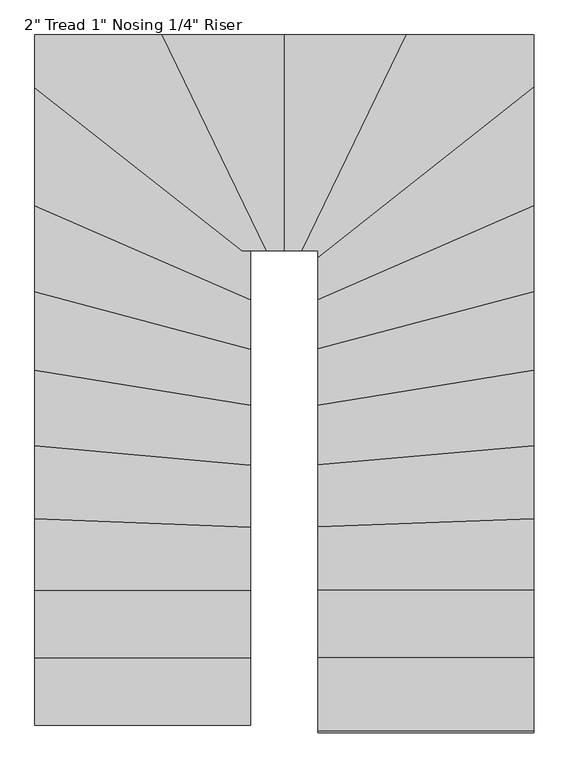
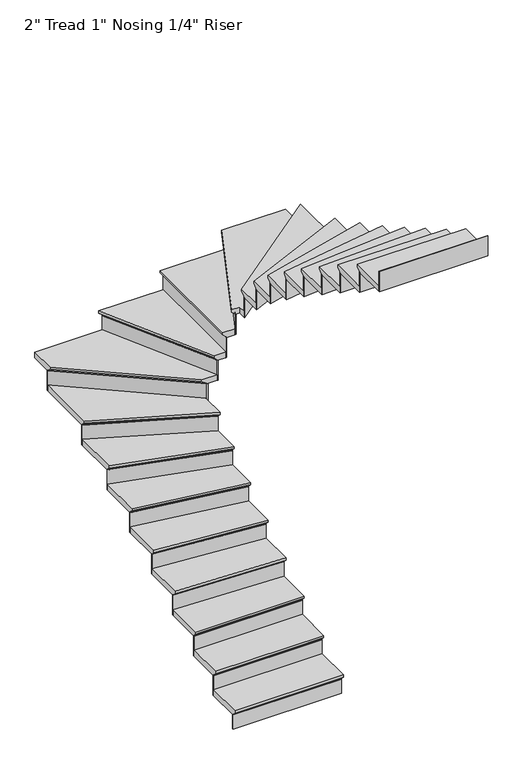
"""IFC4 building model written with IfcOpenShell, lengths in millimetres: stair flight geometry."""

from ifc_helpers import new_model, si_unit, origin, place, context, project, spatial, faceted_brep, source, transform, mapped, element, save


def stair_flight_77a7b7b7(model_context):
    return source(origin(), model_context, "Body", "Brep", [
        faceted_brep([(-5047.1987704, -4554.2130548, 25758.3214286), (-5047.1987704, -4554.2130548, 25777.3714286), (-5940.8822214, -4554.2130548, 25777.3714286), (-5940.8822214, -4554.2130548, 25758.3214286), (-5047.1987704, -4528.8130548, 25732.9214286), (-5940.8822214, -4528.8130548, 25732.9214286), (-5047.1987704, -4249.4130548, 25777.3714286), (-5940.8822214, -4249.4130548, 25777.3714286), (-5940.8822214, -4528.8130548, 25726.5714286), (-5940.8822214, -4249.4130548, 25726.5714286), (-5047.1987704, -4249.4130548, 25726.5714286), (-5047.1987704, -4528.8130548, 25726.5714286)], [[[0, 1, 2, 3]], [[4, 0, 3, 5]], [[2, 1, 6, 7]], [[8, 9, 10, 11]], [[2, 7, 9, 8, 5, 3]], [[8, 11, 4, 5]], [[6, 1, 0, 4, 11, 10]], [[7, 6, 10, 9]]]),
        faceted_brep([(-5047.1987704, -4528.8130548, 25726.5714286), (-5047.1987704, -4528.8130548, 25603.2), (-5047.1987704, -4522.4630548, 25603.2), (-5047.1987704, -4522.4630548, 25726.5714286), (-5940.8822214, -4528.8130548, 25726.5714286), (-5940.8822214, -4522.4630548, 25726.5714286), (-5940.8822214, -4522.4630548, 25603.2), (-5940.8822214, -4528.8130548, 25603.2)], [[[0, 1, 2, 3]], [[4, 5, 6, 7]], [[1, 0, 4, 7]], [[2, 1, 7, 6]], [[3, 2, 6, 5]], [[0, 3, 5, 4]]]),
        faceted_brep([(-5047.1987704, -4249.4130548, 25900.7428571), (-5047.1987704, -4249.4130548, 25726.5714286), (-5047.1987704, -4243.0630548, 25726.5714286), (-5047.1987704, -4243.0630548, 25900.7428571), (-5940.8822214, -4249.4130548, 25900.7428571), (-5940.8822214, -4243.0630548, 25900.7428571), (-5940.8822214, -4243.0630548, 25726.5714286), (-5940.8822214, -4249.4130548, 25726.5714286)], [[[0, 1, 2, 3]], [[4, 5, 6, 7]], [[1, 0, 4, 7]], [[2, 1, 7, 6]], [[3, 2, 6, 5]], [[0, 3, 5, 4]]]),
        faceted_brep([(-5940.8822214, -4274.8130548, 25951.5428571), (-5047.1987704, -4274.8130548, 25951.5428571), (-5047.1987704, -3970.0130548, 25951.5428571), (-5940.8822214, -3970.0130548, 25951.5428571), (-5940.8822214, -4249.4130548, 25900.7428571), (-5940.8822214, -3970.0130548, 25900.7428571), (-5047.1987704, -3970.0130548, 25900.7428571), (-5047.1987704, -4249.4130548, 25900.7428571), (-5940.8822214, -4249.4130548, 25907.0928571), (-5940.8822214, -4274.8130548, 25932.4928571), (-5047.1987704, -4249.4130548, 25907.0928571), (-5047.1987704, -4274.8130548, 25932.4928571)], [[[0, 1, 2, 3]], [[4, 5, 6, 7]], [[0, 3, 5, 4, 8, 9]], [[4, 7, 10, 8]], [[2, 1, 11, 10, 7, 6]], [[3, 2, 6, 5]], [[11, 1, 0, 9]], [[10, 11, 9, 8]]]),
        faceted_brep([(-5047.1987704, -3970.0130548, 26074.9142857), (-5047.1987704, -3970.0130548, 25900.7428571), (-5047.1987704, -3963.6630548, 25900.7428571), (-5047.1987704, -3963.6630548, 26074.9142857), (-5940.8822214, -3970.0130548, 26074.9142857), (-5940.8822214, -3963.6630548, 26074.9142857), (-5940.8822214, -3963.6630548, 25900.7428571), (-5940.8822214, -3970.0130548, 25900.7428571)], [[[0, 1, 2, 3]], [[4, 5, 6, 7]], [[1, 0, 4, 7]], [[2, 1, 7, 6]], [[3, 2, 6, 5]], [[0, 3, 5, 4]]]),
        faceted_brep([(-5940.8822214, -3995.4130548, 26125.7142857), (-5047.1987704, -3995.4130548, 26125.7142857), (-5047.1987704, -3707.9036879, 26125.7142857), (-5940.8822214, -3673.2843203, 26125.7142857), (-5940.8822214, -3970.0130548, 26074.9142857), (-5940.8822214, -3673.2843203, 26074.9142857), (-5047.1987704, -3707.9036879, 26074.9142857), (-5047.1987704, -3970.0130548, 26074.9142857), (-5940.8822214, -3970.0130548, 26081.2642857), (-5940.8822214, -3995.4130548, 26106.6642857), (-5047.1987704, -3970.0130548, 26081.2642857), (-5047.1987704, -3995.4130548, 26106.6642857)], [[[0, 1, 2, 3]], [[4, 5, 6, 7]], [[0, 3, 5, 4, 8, 9]], [[4, 7, 10, 8]], [[2, 1, 11, 10, 7, 6]], [[3, 2, 6, 5]], [[11, 1, 0, 9]], [[10, 11, 9, 8]]]),
        faceted_brep([(-5047.1987704, -3707.9036879, 26249.0857143), (-5047.1987704, -3707.9036879, 26074.9142857), (-5047.1987704, -3701.5489252, 26074.9142857), (-5047.1987704, -3701.5489252, 26249.0857143), (-5940.8822214, -3673.2843203, 26249.0857143), (-5940.8822214, -3666.9295576, 26249.0857143), (-5940.8822214, -3666.9295576, 26074.9142857), (-5940.8822214, -3673.2843203, 26074.9142857)], [[[0, 1, 2, 3]], [[4, 5, 6, 7]], [[1, 0, 4, 7]], [[2, 1, 7, 6]], [[3, 2, 6, 5]], [[0, 3, 5, 4]]]),
        faceted_brep([(-5940.8822214, -3698.703371, 26299.8857143), (-5047.1987704, -3733.3227386, 26299.8857143), (-5047.1987704, -3451.3234819, 26299.8857143), (-5940.8822214, -3370.89733, 26299.8857143), (-5940.8822214, -3673.2843203, 26249.0857143), (-5940.8822214, -3370.89733, 26249.0857143), (-5047.1987704, -3451.3234819, 26249.0857143), (-5047.1987704, -3707.9036879, 26249.0857143), (-5940.8822214, -3673.2843203, 26255.4357143), (-5940.8822214, -3698.703371, 26280.8357143), (-5047.1987704, -3707.9036879, 26255.4357143), (-5047.1987704, -3733.3227386, 26280.8357143)], [[[0, 1, 2, 3]], [[4, 5, 6, 7]], [[0, 3, 5, 4, 8, 9]], [[4, 7, 10, 8]], [[2, 1, 11, 10, 7, 6]], [[3, 2, 6, 5]], [[11, 1, 0, 9]], [[10, 11, 9, 8]]]),
        faceted_brep([(-5047.1987704, -3451.3234819, 26423.2571429), (-5047.1987704, -3451.3234819, 26249.0857143), (-5047.1987704, -3444.9478197, 26249.0857143), (-5047.1987704, -3444.9478197, 26423.2571429), (-5940.8822214, -3370.89733, 26423.2571429), (-5940.8822214, -3364.5216678, 26423.2571429), (-5940.8822214, -3364.5216678, 26249.0857143), (-5940.8822214, -3370.89733, 26249.0857143)], [[[0, 1, 2, 3]], [[4, 5, 6, 7]], [[1, 0, 4, 7]], [[2, 1, 7, 6]], [[3, 2, 6, 5]], [[0, 3, 5, 4]]]),
        faceted_brep([(-5940.8822214, -3396.3999789, 26474.0571429), (-5047.1987704, -3476.8261308, 26474.0571429), (-5047.1987704, -3203.4301079, 26474.0571429), (-5940.8822214, -3059.5417727, 26474.0571429), (-5940.8822214, -3370.89733, 26423.2571429), (-5940.8822214, -3059.5417727, 26423.2571429), (-5047.1987704, -3203.4301079, 26423.2571429), (-5047.1987704, -3451.3234819, 26423.2571429), (-5940.8822214, -3370.89733, 26429.6071429), (-5940.8822214, -3396.3999789, 26455.0071429), (-5047.1987704, -3451.3234819, 26429.6071429), (-5047.1987704, -3476.8261308, 26455.0071429)], [[[0, 1, 2, 3]], [[4, 5, 6, 7]], [[0, 3, 5, 4, 8, 9]], [[4, 7, 10, 8]], [[2, 1, 11, 10, 7, 6]], [[3, 2, 6, 5]], [[11, 1, 0, 9]], [[10, 11, 9, 8]]]),
        faceted_brep([(-5047.1987704, -3203.4301079, 26597.4285714), (-5047.1987704, -3203.4301079, 26423.2571429), (-5047.1987704, -3196.9983292, 26423.2571429), (-5047.1987704, -3196.9983292, 26597.4285714), (-5940.8822214, -3059.5417727, 26597.4285714), (-5940.8822214, -3053.109994, 26597.4285714), (-5940.8822214, -3053.109994, 26423.2571429), (-5940.8822214, -3059.5417727, 26423.2571429)], [[[0, 1, 2, 3]], [[4, 5, 6, 7]], [[1, 0, 4, 7]], [[2, 1, 7, 6]], [[3, 2, 6, 5]], [[0, 3, 5, 4]]]),
        faceted_brep([(-5940.8822214, -3085.2688872, 26648.2285714), (-5047.1987704, -3229.1572224, 26648.2285714), (-5047.1987704, -2970.3553609, 26648.2285714), (-5940.8822214, -2732.7052783, 26648.2285714), (-5940.8822214, -3059.5417727, 26597.4285714), (-5940.8822214, -2732.7052783, 26597.4285714), (-5047.1987704, -2970.3553609, 26597.4285714), (-5047.1987704, -3203.4301079, 26597.4285714), (-5940.8822214, -3059.5417727, 26603.7785714), (-5940.8822214, -3085.2688872, 26629.1785714), (-5047.1987704, -3203.4301079, 26603.7785714), (-5047.1987704, -3229.1572224, 26629.1785714)], [[[0, 1, 2, 3]], [[4, 5, 6, 7]], [[0, 3, 5, 4, 8, 9]], [[4, 7, 10, 8]], [[2, 1, 11, 10, 7, 6]], [[3, 2, 6, 5]], [[11, 1, 0, 9]], [[10, 11, 9, 8]]]),
        faceted_brep([(-5047.1987704, -2970.3553609, 26771.6), (-5047.1987704, -2970.3553609, 26597.4285714), (-5047.1987704, -2963.7846771, 26597.4285714), (-5047.1987704, -2963.7846771, 26771.6), (-5940.8822214, -2732.7052783, 26771.6), (-5940.8822214, -2726.1345945, 26771.6), (-5940.8822214, -2726.1345945, 26597.4285714), (-5940.8822214, -2732.7052783, 26597.4285714)], [[[0, 1, 2, 3]], [[4, 5, 6, 7]], [[1, 0, 4, 7]], [[2, 1, 7, 6]], [[3, 2, 6, 5]], [[0, 3, 5, 4]]]),
        faceted_brep([(-5940.8822214, -2758.9880136, 26822.4), (-5047.1987704, -2996.6380961, 26822.4), (-5047.1987704, -2765.8050203, 26822.4), (-5940.8822214, -2375.5896532, 26822.4), (-5940.8822214, -2732.7052783, 26771.6), (-5940.8822214, -2375.5896532, 26771.6), (-5047.1987704, -2765.8050203, 26771.6), (-5047.1987704, -2970.3553609, 26771.6), (-5940.8822214, -2732.7052783, 26777.95), (-5940.8822214, -2758.9880136, 26803.35), (-5047.1987704, -2970.3553609, 26777.95), (-5047.1987704, -2996.6380961, 26803.35)], [[[0, 1, 2, 3]], [[4, 5, 6, 7]], [[0, 3, 5, 4, 8, 9]], [[4, 7, 10, 8]], [[2, 1, 11, 10, 7, 6]], [[3, 2, 6, 5]], [[11, 1, 0, 9]], [[10, 11, 9, 8]]]),
        faceted_brep([(-5047.1987704, -2765.8050203, 26945.7714286), (-5047.1987704, -2765.8050203, 26771.6), (-5047.1987704, -2758.8760908, 26771.6), (-5047.1987704, -2758.8760908, 26945.7714286), (-5940.8822214, -2375.5896532, 26945.7714286), (-5940.8822214, -2368.6607237, 26945.7714286), (-5940.8822214, -2368.6607237, 26771.6), (-5940.8822214, -2375.5896532, 26771.6)], [[[0, 1, 2, 3]], [[4, 5, 6, 7]], [[1, 0, 4, 7]], [[2, 1, 7, 6]], [[3, 2, 6, 5]], [[0, 3, 5, 4]]]),
        faceted_brep([(-5940.8822214, -2403.3053713, 26996.5714286), (-5047.1987704, -2793.5207384, 26996.5714286), (-5047.1987704, -2590.8424524, 26996.5714286), (-5040.8038639, -2590.8424524, 26996.5714286), (-5940.8822214, -1882.1944717, 26996.5714286), (-5940.8822214, -2375.5896532, 26945.7714286), (-5940.8822214, -1882.1944717, 26945.7714286), (-5040.8038639, -2590.8424524, 26945.7714286), (-5047.1987704, -2590.8424524, 26945.7714286), (-5047.1987704, -2765.8050203, 26945.7714286), (-5940.8822214, -2375.5896532, 26952.1214286), (-5940.8822214, -2403.3053713, 26977.5214286), (-5047.1987704, -2765.8050203, 26952.1214286), (-5047.1987704, -2793.5207384, 26977.5214286)], [[[0, 1, 2, 3, 4]], [[5, 6, 7, 8, 9]], [[0, 4, 6, 5, 10, 11]], [[5, 9, 12, 10]], [[2, 1, 13, 12, 9, 8]], [[4, 3, 7, 6]], [[13, 1, 0, 11]], [[12, 13, 11, 10]], [[3, 2, 8, 7]]]),
        faceted_brep([(-5040.8038639, -2590.8424524, 27119.9428571), (-5040.8038639, -2590.8424524, 26945.7714286), (-5030.5387554, -2590.8424524, 26945.7714286), (-5030.5387554, -2590.8424524, 27119.9428571), (-5940.8822214, -1882.1944717, 27119.9428571), (-5940.8822214, -1874.1125661, 27119.9428571), (-5940.8822214, -1874.1125661, 26945.7714286), (-5940.8822214, -1882.1944717, 26945.7714286)], [[[0, 1, 2, 3]], [[4, 5, 6, 7]], [[1, 0, 4, 7]], [[2, 1, 7, 6]], [[3, 2, 6, 5]], [[0, 3, 5, 4]]]),
        faceted_brep([(-5384.6489457, -1697.1590014, 27170.7428571), (-5940.8822214, -1697.1590014, 27170.7428571), (-5940.8822214, -1914.5220945, 27170.7428571), (-5081.8642978, -2590.8424524, 27170.7428571), (-4952.3566185, -2590.8424524, 27170.7428571), (-5940.8822214, -1697.1590014, 27119.9428571), (-5384.6489457, -1697.1590014, 27119.9428571), (-4952.3566185, -2590.8424524, 27119.9428571), (-5040.8038639, -2590.8424524, 27119.9428571), (-5940.8822214, -1882.1944717, 27119.9428571), (-5940.8822214, -1882.1944717, 27126.2928571), (-5940.8822214, -1914.5220945, 27151.6928571), (-5040.8038639, -2590.8424524, 27126.2928571), (-5081.8642978, -2590.8424524, 27151.6928571)], [[[0, 1, 2, 3, 4]], [[5, 6, 7, 8, 9]], [[1, 0, 6, 5]], [[2, 1, 5, 9, 10, 11]], [[9, 8, 12, 10]], [[4, 3, 13, 12, 8, 7]], [[0, 4, 7, 6]], [[13, 3, 2, 11]], [[12, 13, 11, 10]]]),
        faceted_brep([(-4952.3566185, -2590.8424524, 27294.1142857), (-4952.3566185, -2590.8424524, 27119.9428571), (-4945.3027294, -2590.8424524, 27119.9428571), (-4945.3027294, -2590.8424524, 27294.1142857), (-5384.6489457, -1697.1590014, 27294.1142857), (-5377.5950566, -1697.1590014, 27294.1142857), (-5377.5950566, -1697.1590014, 27119.9428571), (-5384.6489457, -1697.1590014, 27119.9428571)], [[[0, 1, 2, 3]], [[4, 5, 6, 7]], [[1, 0, 4, 7]], [[2, 1, 7, 6]], [[3, 2, 6, 5]], [[0, 3, 5, 4]]]),
        faceted_brep([(-5412.8645022, -1697.1590014, 27344.9142857), (-4980.5721749, -2590.8424524, 27344.9142857), (-4882.0987704, -2590.8424524, 27344.9142857), (-4882.0987706, -1697.1590014, 27344.9142857), (-5384.6489457, -1697.1590014, 27294.1142857), (-4882.0987706, -1697.1590014, 27294.1142857), (-4882.0987704, -2590.8424524, 27294.1142857), (-4952.3566185, -2590.8424524, 27294.1142857), (-5384.6489457, -1697.1590014, 27300.4642857), (-5412.8645022, -1697.1590014, 27325.8642857), (-4952.3566185, -2590.8424524, 27300.4642857), (-4980.5721749, -2590.8424524, 27325.8642857)], [[[0, 1, 2, 3]], [[4, 5, 6, 7]], [[0, 3, 5, 4, 8, 9]], [[4, 7, 10, 8]], [[3, 2, 6, 5]], [[11, 1, 0, 9]], [[10, 11, 9, 8]], [[2, 1, 11, 10, 7, 6]]]),
        faceted_brep([(-4882.0987704, -2590.8424524, 27468.2857143), (-4882.0987704, -2590.8424524, 27294.1142857), (-4875.7487704, -2590.8424524, 27294.1142857), (-4875.7487704, -2590.8424524, 27468.2857143), (-4882.0987706, -1697.1590014, 27468.2857143), (-4875.7487706, -1697.1590014, 27468.2857143), (-4875.7487706, -1697.1590014, 27294.1142857), (-4882.0987706, -1697.1590014, 27294.1142857)], [[[0, 1, 2, 3]], [[4, 5, 6, 7]], [[1, 0, 4, 7]], [[2, 1, 7, 6]], [[3, 2, 6, 5]], [[0, 3, 5, 4]]]),
        faceted_brep([(-4907.4987706, -1697.1590014, 27519.0857143), (-4907.4987704, -2590.8424524, 27519.0857143), (-4806.2098095, -2590.8424524, 27519.0857143), (-4373.9174828, -1697.1590014, 27519.0857143), (-4882.0987706, -1697.1590014, 27468.2857143), (-4373.9174828, -1697.1590014, 27468.2857143), (-4806.2098095, -2590.8424524, 27468.2857143), (-4882.0987704, -2590.8424524, 27468.2857143), (-4882.0987706, -1697.1590014, 27474.6357143), (-4907.4987706, -1697.1590014, 27500.0357143), (-4882.0987704, -2590.8424524, 27474.6357143), (-4907.4987704, -2590.8424524, 27500.0357143)], [[[0, 1, 2, 3]], [[4, 5, 6, 7]], [[0, 3, 5, 4, 8, 9]], [[4, 7, 10, 8]], [[2, 1, 11, 10, 7, 6]], [[3, 2, 6, 5]], [[11, 1, 0, 9]], [[10, 11, 9, 8]]]),
        faceted_brep([(-4806.2098095, -2590.8424524, 27642.4571429), (-4806.2098095, -2590.8424524, 27468.2857143), (-4799.1559204, -2590.8424524, 27468.2857143), (-4799.1559204, -2590.8424524, 27642.4571429), (-4373.9174828, -1697.1590014, 27642.4571429), (-4366.8635937, -1697.1590014, 27642.4571429), (-4366.8635937, -1697.1590014, 27468.2857143), (-4373.9174828, -1697.1590014, 27468.2857143)], [[[0, 1, 2, 3]], [[4, 5, 6, 7]], [[1, 0, 4, 7]], [[2, 1, 7, 6]], [[3, 2, 6, 5]], [[0, 3, 5, 4]]]),
        faceted_brep([(-3874.1153195, -1946.8497166, 27693.2571429), (-3874.1153195, -1697.1590014, 27693.2571429), (-4402.1330392, -1697.1590014, 27693.2571429), (-4834.4253659, -2590.8424524, 27693.2571429), (-4767.7987704, -2590.8424524, 27693.2571429), (-4767.7987704, -2650.4628721, 27693.2571429), (-3874.1153195, -1697.1590014, 27642.4571429), (-3874.1153195, -1946.8497166, 27642.4571429), (-4767.7987704, -2650.4628721, 27642.4571429), (-4767.7987704, -2590.8424524, 27642.4571429), (-4806.2098095, -2590.8424524, 27642.4571429), (-4373.9174828, -1697.1590014, 27642.4571429), (-4806.2098095, -2590.8424524, 27648.8071429), (-4373.9174828, -1697.1590014, 27648.8071429), (-4834.4253659, -2590.8424524, 27674.2071429), (-4402.1330392, -1697.1590014, 27674.2071429)], [[[0, 1, 2, 3, 4, 5]], [[6, 7, 8, 9, 10, 11]], [[1, 0, 7, 6]], [[11, 10, 12, 13]], [[4, 3, 14, 12, 10, 9]], [[5, 4, 9, 8]], [[0, 5, 8, 7]], [[14, 3, 2, 15]], [[12, 14, 15, 13]], [[2, 1, 6, 11, 13, 15]]]),
        faceted_brep([(-4767.7987704, -2650.4628721, 27816.6285714), (-4767.7987704, -2650.4628721, 27642.4571429), (-4767.7987704, -2658.5447778, 27642.4571429), (-4767.7987704, -2658.5447778, 27816.6285714), (-3874.1153195, -1946.8497166, 27816.6285714), (-3874.1153195, -1954.9316222, 27816.6285714), (-3874.1153195, -1954.9316222, 27642.4571429), (-3874.1153195, -1946.8497166, 27642.4571429)], [[[0, 1, 2, 3]], [[4, 5, 6, 7]], [[1, 0, 4, 7]], [[2, 1, 7, 6]], [[3, 2, 6, 5]], [[0, 3, 5, 4]]]),
        faceted_brep([(-3874.1153195, -1914.5220938, 27867.4285714), (-4767.7987704, -2618.1352494, 27867.4285714), (-4767.7987704, -2821.2364563, 27867.4285714), (-3874.1153195, -2431.0210889, 27867.4285714), (-3874.1153195, -1946.8497166, 27816.6285714), (-3874.1153195, -2431.0210889, 27816.6285714), (-4767.7987704, -2821.2364563, 27816.6285714), (-4767.7987704, -2650.4628721, 27816.6285714), (-3874.1153195, -1946.8497166, 27822.9785714), (-3874.1153195, -1914.5220938, 27848.3785714), (-4767.7987704, -2650.4628721, 27822.9785714), (-4767.7987704, -2618.1352494, 27848.3785714)], [[[0, 1, 2, 3]], [[4, 5, 6, 7]], [[0, 3, 5, 4, 8, 9]], [[4, 7, 10, 8]], [[2, 1, 11, 10, 7, 6]], [[3, 2, 6, 5]], [[11, 1, 0, 9]], [[10, 11, 9, 8]]]),
        faceted_brep([(-4767.7987704, -2821.2364563, 27990.8), (-4767.7987704, -2821.2364563, 27816.6285714), (-4767.7987704, -2828.1653858, 27816.6285714), (-4767.7987704, -2828.1653858, 27990.8), (-3874.1153195, -2431.0210889, 27990.8), (-3874.1153195, -2437.9500185, 27990.8), (-3874.1153195, -2437.9500185, 27816.6285714), (-3874.1153195, -2431.0210889, 27816.6285714)], [[[0, 1, 2, 3]], [[4, 5, 6, 7]], [[1, 0, 4, 7]], [[2, 1, 7, 6]], [[3, 2, 6, 5]], [[0, 3, 5, 4]]]),
        faceted_brep([(-3874.1153195, -2403.3053709, 28041.6), (-4767.7987704, -2793.5207382, 28041.6), (-4767.7987704, -3022.9208311, 28041.6), (-3874.1153195, -2785.2707484, 28041.6), (-3874.1153195, -2431.0210889, 27990.8), (-3874.1153195, -2785.2707484, 27990.8), (-4767.7987704, -3022.9208311, 27990.8), (-4767.7987704, -2821.2364563, 27990.8), (-3874.1153195, -2431.0210889, 27997.15), (-3874.1153195, -2403.3053709, 28022.55), (-4767.7987704, -2821.2364563, 27997.15), (-4767.7987704, -2793.5207382, 28022.55)], [[[0, 1, 2, 3]], [[4, 5, 6, 7]], [[0, 3, 5, 4, 8, 9]], [[4, 7, 10, 8]], [[2, 1, 11, 10, 7, 6]], [[3, 2, 6, 5]], [[11, 1, 0, 9]], [[10, 11, 9, 8]]]),
        faceted_brep([(-4767.7987704, -3022.9208311, 28164.9714286), (-4767.7987704, -3022.9208311, 27990.8), (-4767.7987704, -3029.4915149, 27990.8), (-4767.7987704, -3029.4915149, 28164.9714286), (-3874.1153195, -2785.2707484, 28164.9714286), (-3874.1153195, -2791.8414322, 28164.9714286), (-3874.1153195, -2791.8414322, 27990.8), (-3874.1153195, -2785.2707484, 27990.8)], [[[0, 1, 2, 3]], [[4, 5, 6, 7]], [[1, 0, 4, 7]], [[2, 1, 7, 6]], [[3, 2, 6, 5]], [[0, 3, 5, 4]]]),
        faceted_brep([(-3874.1153195, -2758.9880132, 28215.7714286), (-4767.7987704, -2996.6380959, 28215.7714286), (-4767.7987704, -3254.8843368, 28215.7714286), (-3874.1153195, -3110.9960015, 28215.7714286), (-3874.1153195, -2785.2707484, 28164.9714286), (-3874.1153195, -3110.9960015, 28164.9714286), (-4767.7987704, -3254.8843368, 28164.9714286), (-4767.7987704, -3022.9208311, 28164.9714286), (-3874.1153195, -2785.2707484, 28171.3214286), (-3874.1153195, -2758.9880132, 28196.7214286), (-4767.7987704, -3022.9208311, 28171.3214286), (-4767.7987704, -2996.6380959, 28196.7214286)], [[[0, 1, 2, 3]], [[4, 5, 6, 7]], [[0, 3, 5, 4, 8, 9]], [[4, 7, 10, 8]], [[2, 1, 11, 10, 7, 6]], [[3, 2, 6, 5]], [[11, 1, 0, 9]], [[10, 11, 9, 8]]]),
        faceted_brep([(-4767.7987704, -3254.8843368, 28339.1428571), (-4767.7987704, -3254.8843368, 28164.9714286), (-4767.7987704, -3261.3161154, 28164.9714286), (-4767.7987704, -3261.3161154, 28339.1428571), (-3874.1153195, -3110.9960015, 28339.1428571), (-3874.1153195, -3117.4277801, 28339.1428571), (-3874.1153195, -3117.4277801, 28164.9714286), (-3874.1153195, -3110.9960015, 28164.9714286)], [[[0, 1, 2, 3]], [[4, 5, 6, 7]], [[1, 0, 4, 7]], [[2, 1, 7, 6]], [[3, 2, 6, 5]], [[0, 3, 5, 4]]]),
        faceted_brep([(-3874.1153195, -3085.2688869, 28389.9428571), (-4767.7987704, -3229.1572222, 28389.9428571), (-4767.7987704, -3502.3287795, 28389.9428571), (-3874.1153195, -3421.9026274, 28389.9428571), (-3874.1153195, -3110.9960015, 28339.1428571), (-3874.1153195, -3421.9026274, 28339.1428571), (-4767.7987704, -3502.3287795, 28339.1428571), (-4767.7987704, -3254.8843368, 28339.1428571), (-3874.1153195, -3110.9960015, 28345.4928571), (-3874.1153195, -3085.2688869, 28370.8928571), (-4767.7987704, -3254.8843368, 28345.4928571), (-4767.7987704, -3229.1572222, 28370.8928571)], [[[0, 1, 2, 3]], [[4, 5, 6, 7]], [[0, 3, 5, 4, 8, 9]], [[4, 7, 10, 8]], [[2, 1, 11, 10, 7, 6]], [[3, 2, 6, 5]], [[11, 1, 0, 9]], [[10, 11, 9, 8]]]),
        faceted_brep([(-4767.7987704, -3502.3287795, 28513.3142857), (-4767.7987704, -3502.3287795, 28339.1428571), (-4767.7987704, -3508.7044417, 28339.1428571), (-4767.7987704, -3508.7044417, 28513.3142857), (-3874.1153195, -3421.9026274, 28513.3142857), (-3874.1153195, -3428.2782897, 28513.3142857), (-3874.1153195, -3428.2782897, 28339.1428571), (-3874.1153195, -3421.9026274, 28339.1428571)], [[[0, 1, 2, 3]], [[4, 5, 6, 7]], [[1, 0, 4, 7]], [[2, 1, 7, 6]], [[3, 2, 6, 5]], [[0, 3, 5, 4]]]),
        faceted_brep([(-3874.1153195, -3396.3999786, 28564.1142857), (-4767.7987704, -3476.8261306, 28564.1142857), (-4767.7987704, -3758.7417891, 28564.1142857), (-3874.1153195, -3724.1224215, 28564.1142857), (-3874.1153195, -3421.9026274, 28513.3142857), (-3874.1153195, -3724.1224215, 28513.3142857), (-4767.7987704, -3758.7417891, 28513.3142857), (-4767.7987704, -3502.3287795, 28513.3142857), (-3874.1153195, -3421.9026274, 28519.6642857), (-3874.1153195, -3396.3999786, 28545.0642857), (-4767.7987704, -3502.3287795, 28519.6642857), (-4767.7987704, -3476.8261306, 28545.0642857)], [[[0, 1, 2, 3]], [[4, 5, 6, 7]], [[0, 3, 5, 4, 8, 9]], [[4, 7, 10, 8]], [[2, 1, 11, 10, 7, 6]], [[3, 2, 6, 5]], [[11, 1, 0, 9]], [[10, 11, 9, 8]]]),
        faceted_brep([(-4767.7987704, -3758.7417891, 28687.4857143), (-4767.7987704, -3758.7417891, 28513.3142857), (-4767.7987704, -3765.0965518, 28513.3142857), (-4767.7987704, -3765.0965518, 28687.4857143), (-3874.1153195, -3724.1224215, 28687.4857143), (-3874.1153195, -3730.4771842, 28687.4857143), (-3874.1153195, -3730.4771842, 28513.3142857), (-3874.1153195, -3724.1224215, 28513.3142857)], [[[0, 1, 2, 3]], [[4, 5, 6, 7]], [[1, 0, 4, 7]], [[2, 1, 7, 6]], [[3, 2, 6, 5]], [[0, 3, 5, 4]]]),
        faceted_brep([(-3874.1153195, -3698.7033708, 28738.2857143), (-4767.7987704, -3733.3227384, 28738.2857143), (-4767.7987704, -4020.8130546, 28738.2857143), (-3874.1153195, -4020.8130546, 28738.2857143), (-3874.1153195, -3724.1224215, 28687.4857143), (-3874.1153195, -4020.8130546, 28687.4857143), (-4767.7987704, -4020.8130546, 28687.4857143), (-4767.7987704, -3758.7417891, 28687.4857143), (-3874.1153195, -3724.1224215, 28693.8357143), (-3874.1153195, -3698.7033708, 28719.2357143), (-4767.7987704, -3758.7417891, 28693.8357143), (-4767.7987704, -3733.3227384, 28719.2357143)], [[[0, 1, 2, 3]], [[4, 5, 6, 7]], [[0, 3, 5, 4, 8, 9]], [[4, 7, 10, 8]], [[2, 1, 11, 10, 7, 6]], [[3, 2, 6, 5]], [[11, 1, 0, 9]], [[10, 11, 9, 8]]]),
        faceted_brep([(-4767.7987704, -4020.8130546, 28861.6571429), (-4767.7987704, -4020.8130546, 28687.4857143), (-4767.7987704, -4027.1630546, 28687.4857143), (-4767.7987704, -4027.1630546, 28861.6571429), (-3874.1153195, -4020.8130546, 28861.6571429), (-3874.1153195, -4027.1630546, 28861.6571429), (-3874.1153195, -4027.1630546, 28687.4857143), (-3874.1153195, -4020.8130546, 28687.4857143)], [[[0, 1, 2, 3]], [[4, 5, 6, 7]], [[1, 0, 4, 7]], [[2, 1, 7, 6]], [[3, 2, 6, 5]], [[0, 3, 5, 4]]]),
        faceted_brep([(-3874.1153195, -3995.4130546, 28912.4571429), (-4767.7987704, -3995.4130546, 28912.4571429), (-4767.7987704, -4300.2130546, 28912.4571429), (-3874.1153195, -4300.2130546, 28912.4571429), (-3874.1153195, -4020.8130546, 28861.6571429), (-3874.1153195, -4300.2130546, 28861.6571429), (-4767.7987704, -4300.2130546, 28861.6571429), (-4767.7987704, -4020.8130546, 28861.6571429), (-3874.1153195, -4020.8130546, 28868.0071429), (-3874.1153195, -3995.4130546, 28893.4071429), (-4767.7987704, -4020.8130546, 28868.0071429), (-4767.7987704, -3995.4130546, 28893.4071429)], [[[0, 1, 2, 3]], [[4, 5, 6, 7]], [[0, 3, 5, 4, 8, 9]], [[4, 7, 10, 8]], [[2, 1, 11, 10, 7, 6]], [[3, 2, 6, 5]], [[11, 1, 0, 9]], [[10, 11, 9, 8]]]),
        faceted_brep([(-4767.7987704, -4300.2130546, 29035.8285714), (-4767.7987704, -4300.2130546, 28861.6571429), (-4767.7987704, -4306.5630546, 28861.6571429), (-4767.7987704, -4306.5630546, 29035.8285714), (-3874.1153195, -4300.2130546, 29035.8285714), (-3874.1153195, -4306.5630546, 29035.8285714), (-3874.1153195, -4306.5630546, 28861.6571429), (-3874.1153195, -4300.2130546, 28861.6571429)], [[[0, 1, 2, 3]], [[4, 5, 6, 7]], [[1, 0, 4, 7]], [[2, 1, 7, 6]], [[3, 2, 6, 5]], [[0, 3, 5, 4]]]),
        faceted_brep([(-4767.7987704, -4579.6130546, 29210.0), (-4767.7987704, -4579.6130546, 29035.8285714), (-4767.7987704, -4585.9630546, 29035.8285714), (-4767.7987704, -4585.9630546, 29210.0), (-3874.1153195, -4579.6130546, 29210.0), (-3874.1153195, -4585.9630546, 29210.0), (-3874.1153195, -4585.9630546, 29035.8285714), (-3874.1153195, -4579.6130546, 29035.8285714)], [[[0, 1, 2, 3]], [[4, 5, 6, 7]], [[1, 0, 4, 7]], [[2, 1, 7, 6]], [[3, 2, 6, 5]], [[0, 3, 5, 4]]]),
        faceted_brep([(-3874.1153195, -4274.8130546, 29086.6285714), (-4767.7987704, -4274.8130546, 29086.6285714), (-4767.7987704, -4579.6130546, 29086.6285714), (-3874.1153195, -4579.6130546, 29086.6285714), (-3874.1153195, -4300.2130546, 29035.8285714), (-3874.1153195, -4579.6130546, 29035.8285714), (-4767.7987704, -4579.6130546, 29035.8285714), (-4767.7987704, -4300.2130546, 29035.8285714), (-3874.1153195, -4300.2130546, 29042.1785714), (-3874.1153195, -4274.8130546, 29067.5785714), (-4767.7987704, -4300.2130546, 29042.1785714), (-4767.7987704, -4274.8130546, 29067.5785714)], [[[0, 1, 2, 3]], [[4, 5, 6, 7]], [[0, 3, 5, 4, 8, 9]], [[4, 7, 10, 8]], [[2, 1, 11, 10, 7, 6]], [[3, 2, 6, 5]], [[11, 1, 0, 9]], [[10, 11, 9, 8]]]),
    ])


if __name__ == "__main__":
    model = new_model("IFC4")
    model_context = context("Model", 3, world=origin())
    ifc_project = project(units=[si_unit("LENGTHUNIT", "METRE", prefix="MILLI")], contexts=[model_context])
    site = spatial("IfcSite", under=ifc_project)
    building = spatial("IfcBuilding", under=site)
    placement = place(None, origin())
    stair_flight_shape = stair_flight_77a7b7b7(model_context)
    element("IfcStairFlight", 1, ObjectType="2\" Tread 1\" Nosing 1/4\" Riser", at=placement, inside=building, context=model_context, shape_type="MappedRepresentation", body=[
        mapped(stair_flight_shape, transform((0.0, 0.0, 0.0), x_axis=(1.0, 0.0, 0.0), y_axis=(0.0, 1.0, 0.0), z_axis=(0.0, 0.0, 1.0))),
    ])
    save(model, "model.ifc")

# Revit data of these elements
# Element 1 (IfcStairFlight, "2\" Tread 1\" Nosing 1/4\" Riser")
#   Materials on its faces: "Tile, Porcelain, 4in"
# Materials
#   "Tile, Porcelain, 4in": class "Generic", colour RGB 89 87 158, transparency 0, Description = "Porcelain tile, 4\", white", Cost = 0
